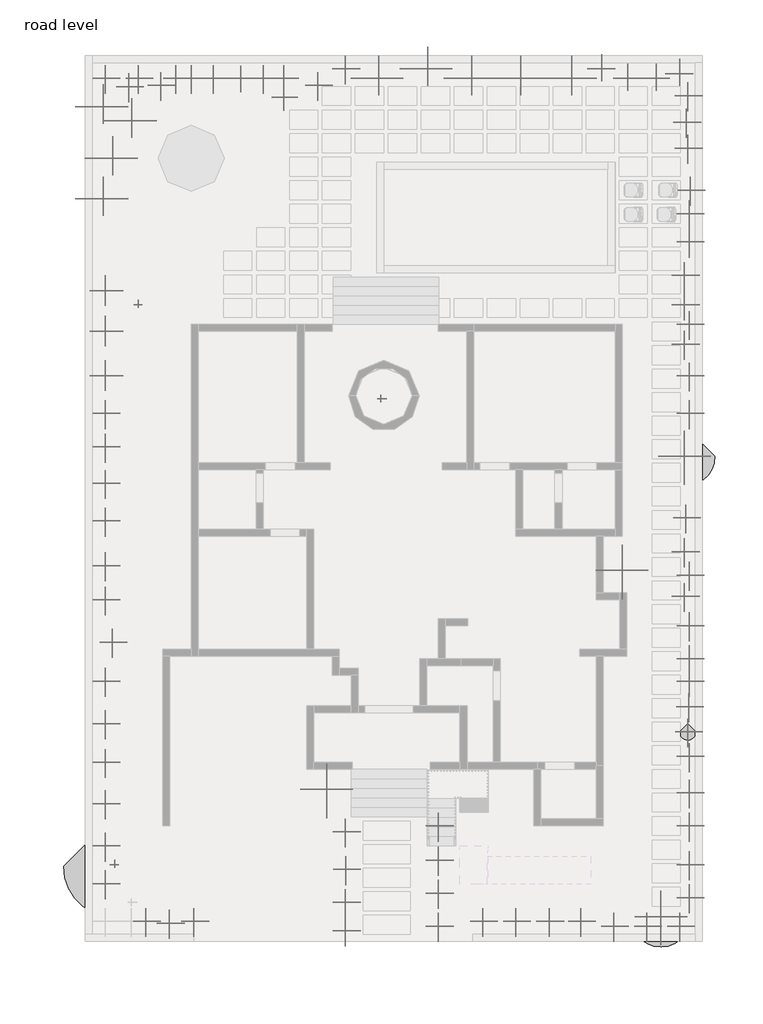
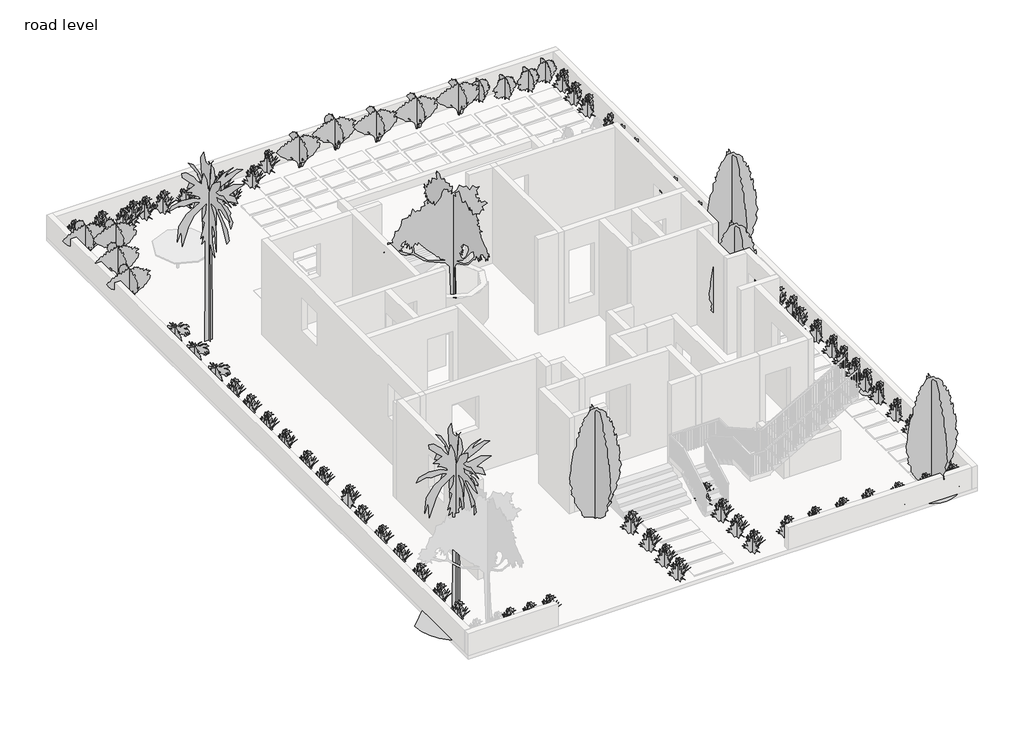
# One storey, part 5 of 5: 93 geographic elements.
"""IFC4 building model written with IfcOpenShell, lengths in millimetres."""

from ifc_helpers import new_model, si_unit, origin, place, context, project, spatial, transform, mapped, element, save
from components import rpc_plant_tropical_55f6ff97, rpc_plant_tropical_6475341c, rpc_plant_tropical_dagger_2_80c14bd7, rpc_plant_tropical_japanese_fern_2_5_30b4c15b, rpc_plant_tropical_jungle_flame_3_9c4808c2, rpc_tree_deciduous_japanese_cherry_15_bc05297b, rpc_tree_tropical_cuban_royal_palm_25_6f0ceb55, rpc_tree_tropical_grass_palm_18_ffc4a38a

model = new_model("IFC4")

# Units and contexts
model_context = context("Model", 3, world=origin())
ifc_project = project(units=[si_unit("LENGTHUNIT", "METRE", prefix="MILLI")], contexts=[model_context])

# Site, building, storey
site = spatial("IfcSite", under=ifc_project)
building = spatial("IfcBuilding", under=site)
storey = spatial("IfcBuildingStorey", under=building, Name="road level", Elevation=0.0)

# Geographic elements
placement = place(None, origin())
rpc_plant_tropical_shape = rpc_plant_tropical_55f6ff97(model_context)
element("IfcGeographicElement", 1, ObjectType="RPC Plant - Tropical", at=placement, inside=storey, context=model_context, shape_type="MappedRepresentation", body=[
    mapped(rpc_plant_tropical_shape, transform((-4250.8487175, 22497.1906886, 0.0), x_axis=(1.0, 0.0, 0.0), y_axis=(0.0, 1.0, 0.0), z_axis=(0.0, 0.0, 1.0))),
])
element("IfcGeographicElement", 2, ObjectType="RPC Plant - Tropical", at=placement, inside=storey, context=model_context, shape_type="MappedRepresentation", body=[
    mapped(rpc_plant_tropical_shape, transform((-3184.0487175, 22497.1906886, 0.0), x_axis=(1.0, 0.0, 0.0), y_axis=(0.0, 1.0, 0.0), z_axis=(0.0, 0.0, 1.0))),
])
element("IfcGeographicElement", 3, ObjectType="RPC Plant - Tropical", at=placement, inside=storey, context=model_context, shape_type="MappedRepresentation", body=[
    mapped(rpc_plant_tropical_shape, transform((-1964.8487175, 22497.1906886, 0.0), x_axis=(1.0, 0.0, 0.0), y_axis=(0.0, 1.0, 0.0), z_axis=(0.0, 0.0, 1.0))),
])
element("IfcGeographicElement", 4, ObjectType="RPC Plant - Tropical", at=placement, inside=storey, context=model_context, shape_type="MappedRepresentation", body=[
    mapped(rpc_plant_tropical_shape, transform((1530.4394971, 22497.1906886, 0.0), x_axis=(1.0, 0.0, 0.0), y_axis=(0.0, 1.0, 0.0), z_axis=(0.0, 0.0, 1.0))),
])
element("IfcGeographicElement", 5, ObjectType="RPC Plant - Tropical", at=placement, inside=storey, context=model_context, shape_type="MappedRepresentation", body=[
    mapped(rpc_plant_tropical_shape, transform((3511.6394971, 22801.9906886, 0.0), x_axis=(1.0, 0.0, 0.0), y_axis=(0.0, 1.0, 0.0), z_axis=(0.0, 0.0, 1.0))),
])
element("IfcGeographicElement", 6, ObjectType="RPC Plant - Tropical", at=placement, inside=storey, context=model_context, shape_type="MappedRepresentation", body=[
    mapped(rpc_plant_tropical_shape, transform((2630.2047352, 22268.5906886, 0.0), x_axis=(1.0, 0.0, 0.0), y_axis=(0.0, 1.0, 0.0), z_axis=(0.0, 0.0, 1.0))),
])
element("IfcGeographicElement", 7, ObjectType="RPC Plant - Tropical", at=placement, inside=storey, context=model_context, shape_type="MappedRepresentation", body=[
    mapped(rpc_plant_tropical_shape, transform((867.2512825, 22497.1906886, 0.0), x_axis=(1.0, 0.0, 0.0), y_axis=(0.0, 1.0, 0.0), z_axis=(0.0, 0.0, 1.0))),
])
element("IfcGeographicElement", 8, ObjectType="RPC Plant - Tropical", at=placement, inside=storey, context=model_context, shape_type="MappedRepresentation", body=[
    mapped(rpc_plant_tropical_shape, transform((-755.5605029, 22497.1906886, 0.0), x_axis=(1.0, 0.0, 0.0), y_axis=(0.0, 1.0, 0.0), z_axis=(0.0, 0.0, 1.0))),
])
element("IfcGeographicElement", 9, ObjectType="RPC Plant - Tropical", at=placement, inside=storey, context=model_context, shape_type="MappedRepresentation", body=[
    mapped(rpc_plant_tropical_shape, transform((-1469.5487175, 22497.1906886, 0.0), x_axis=(1.0, 0.0, 0.0), y_axis=(0.0, 1.0, 0.0), z_axis=(0.0, 0.0, 1.0))),
])
element("IfcGeographicElement", 10, ObjectType="RPC Plant - Tropical", at=placement, inside=storey, context=model_context, shape_type="MappedRepresentation", body=[
    mapped(rpc_plant_tropical_shape, transform((-2459.5797144, 22268.5906886, 0.0), x_axis=(1.0, 0.0, 0.0), y_axis=(0.0, 1.0, 0.0), z_axis=(0.0, 0.0, 1.0))),
])
element("IfcGeographicElement", 11, ObjectType="RPC Plant - Tropical", at=placement, inside=storey, context=model_context, shape_type="MappedRepresentation", body=[
    mapped(rpc_plant_tropical_shape, transform((-3485.1574933, 22224.4169729, 0.0), x_axis=(1.0, 0.0, 0.0), y_axis=(0.0, 1.0, 0.0), z_axis=(0.0, 0.0, 1.0))),
])
element("IfcGeographicElement", 12, ObjectType="RPC Plant - Tropical", at=placement, inside=storey, context=model_context, shape_type="MappedRepresentation", body=[
    mapped(rpc_plant_tropical_shape, transform((14595.9512825, 21938.3906886, 0.0), x_axis=(1.0, 0.0, 0.0), y_axis=(0.0, 1.0, 0.0), z_axis=(0.0, 0.0, 1.0))),
])
element("IfcGeographicElement", 13, ObjectType="RPC Plant - Tropical", at=placement, inside=storey, context=model_context, shape_type="MappedRepresentation", body=[
    mapped(rpc_plant_tropical_shape, transform((14545.1512825, 21074.7906886, 0.0), x_axis=(1.0, 0.0, 0.0), y_axis=(0.0, 1.0, 0.0), z_axis=(0.0, 0.0, 1.0))),
])
element("IfcGeographicElement", 14, ObjectType="RPC Plant - Tropical", at=placement, inside=storey, context=model_context, shape_type="MappedRepresentation", body=[
    mapped(rpc_plant_tropical_shape, transform((14684.8512825, 18877.6906886, 0.0), x_axis=(1.0, 0.0, 0.0), y_axis=(0.0, 1.0, 0.0), z_axis=(0.0, 0.0, 1.0))),
])
element("IfcGeographicElement", 15, ObjectType="RPC Plant - Tropical", at=placement, inside=storey, context=model_context, shape_type="MappedRepresentation", body=[
    mapped(rpc_plant_tropical_shape, transform((14646.7512825, 17201.2906886, 0.0), x_axis=(1.0, 0.0, 0.0), y_axis=(0.0, 1.0, 0.0), z_axis=(0.0, 0.0, 1.0))),
])
element("IfcGeographicElement", 16, ObjectType="RPC Plant - Tropical", at=placement, inside=storey, context=model_context, shape_type="MappedRepresentation", body=[
    mapped(rpc_plant_tropical_shape, transform((14646.7512825, 18115.6906886, 0.0), x_axis=(1.0, 0.0, 0.0), y_axis=(0.0, 1.0, 0.0), z_axis=(0.0, 0.0, 1.0))),
])
element("IfcGeographicElement", 17, ObjectType="RPC Plant - Tropical", at=placement, inside=storey, context=model_context, shape_type="MappedRepresentation", body=[
    mapped(rpc_plant_tropical_shape, transform((14595.9512825, 20236.5906886, 0.0), x_axis=(1.0, 0.0, 0.0), y_axis=(0.0, 1.0, 0.0), z_axis=(0.0, 0.0, 1.0))),
])
element("IfcGeographicElement", 18, ObjectType="RPC Plant - Tropical", at=placement, inside=storey, context=model_context, shape_type="MappedRepresentation", body=[
    mapped(rpc_plant_tropical_shape, transform((14494.3512825, 16121.7906886, 0.0), x_axis=(1.0, 0.0, 0.0), y_axis=(0.0, 1.0, 0.0), z_axis=(0.0, 0.0, 1.0))),
])
element("IfcGeographicElement", 19, ObjectType="RPC Plant - Tropical", at=placement, inside=storey, context=model_context, shape_type="MappedRepresentation", body=[
    mapped(rpc_plant_tropical_shape, transform((14494.3512825, 15169.2906886, 0.0), x_axis=(1.0, 0.0, 0.0), y_axis=(0.0, 1.0, 0.0), z_axis=(0.0, 0.0, 1.0))),
])
element("IfcGeographicElement", 20, ObjectType="RPC Plant - Tropical", at=placement, inside=storey, context=model_context, shape_type="MappedRepresentation", body=[
    mapped(rpc_plant_tropical_shape, transform((14494.3512825, 13898.7232877, 0.0), x_axis=(1.0, 0.0, 0.0), y_axis=(0.0, 1.0, 0.0), z_axis=(0.0, 0.0, 1.0))),
])
element("IfcGeographicElement", 21, ObjectType="RPC Plant - Tropical", at=placement, inside=storey, context=model_context, shape_type="MappedRepresentation", body=[
    mapped(rpc_plant_tropical_shape, transform((14646.7512825, 12870.0232877, 0.0), x_axis=(1.0, 0.0, 0.0), y_axis=(0.0, 1.0, 0.0), z_axis=(0.0, 0.0, 1.0))),
])
element("IfcGeographicElement", 22, ObjectType="RPC Plant - Tropical", at=placement, inside=storey, context=model_context, shape_type="MappedRepresentation", body=[
    mapped(rpc_plant_tropical_shape, transform((14646.7512825, 11650.8232877, 0.0), x_axis=(1.0, 0.0, 0.0), y_axis=(0.0, 1.0, 0.0), z_axis=(0.0, 0.0, 1.0))),
])
element("IfcGeographicElement", 23, ObjectType="RPC Plant - Tropical", at=placement, inside=storey, context=model_context, shape_type="MappedRepresentation", body=[
    mapped(rpc_plant_tropical_shape, transform((-4250.8487175, 11650.8232877, 0.0), x_axis=(1.0, 0.0, 0.0), y_axis=(0.0, 1.0, 0.0), z_axis=(0.0, 0.0, 1.0))),
])
element("IfcGeographicElement", 24, ObjectType="RPC Plant - Tropical", at=placement, inside=storey, context=model_context, shape_type="MappedRepresentation", body=[
    mapped(rpc_plant_tropical_shape, transform((-4250.8487175, 10567.4181776, 0.0), x_axis=(1.0, 0.0, 0.0), y_axis=(0.0, 1.0, 0.0), z_axis=(0.0, 0.0, 1.0))),
])
element("IfcGeographicElement", 25, ObjectType="RPC Plant - Tropical", at=placement, inside=storey, context=model_context, shape_type="MappedRepresentation", body=[
    mapped(rpc_plant_tropical_shape, transform((-4250.8487175, 9390.7906886, 0.0), x_axis=(1.0, 0.0, 0.0), y_axis=(0.0, 1.0, 0.0), z_axis=(0.0, 0.0, 1.0))),
])
element("IfcGeographicElement", 26, ObjectType="RPC Plant - Tropical", at=placement, inside=storey, context=model_context, shape_type="MappedRepresentation", body=[
    mapped(rpc_plant_tropical_shape, transform((-4250.8487175, 8171.5906886, 0.0), x_axis=(1.0, 0.0, 0.0), y_axis=(0.0, 1.0, 0.0), z_axis=(0.0, 0.0, 1.0))),
])
element("IfcGeographicElement", 27, ObjectType="RPC Plant - Tropical", at=placement, inside=storey, context=model_context, shape_type="MappedRepresentation", body=[
    mapped(rpc_plant_tropical_shape, transform((-4250.8487175, 6723.7906886, 0.0), x_axis=(1.0, 0.0, 0.0), y_axis=(0.0, 1.0, 0.0), z_axis=(0.0, 0.0, 1.0))),
])
element("IfcGeographicElement", 28, ObjectType="RPC Plant - Tropical", at=placement, inside=storey, context=model_context, shape_type="MappedRepresentation", body=[
    mapped(rpc_plant_tropical_shape, transform((-4250.8487175, 5618.8906886, 0.0), x_axis=(1.0, 0.0, 0.0), y_axis=(0.0, 1.0, 0.0), z_axis=(0.0, 0.0, 1.0))),
])
element("IfcGeographicElement", 29, ObjectType="RPC Plant - Tropical", at=placement, inside=storey, context=model_context, shape_type="MappedRepresentation", body=[
    mapped(rpc_plant_tropical_shape, transform((-4022.2487175, 4247.2906886, 0.0), x_axis=(1.0, 0.0, 0.0), y_axis=(0.0, 1.0, 0.0), z_axis=(0.0, 0.0, 1.0))),
])
element("IfcGeographicElement", 30, ObjectType="RPC Plant - Tropical", at=placement, inside=storey, context=model_context, shape_type="MappedRepresentation", body=[
    mapped(rpc_plant_tropical_shape, transform((-4250.8487175, 2989.9906886, 0.0), x_axis=(1.0, 0.0, 0.0), y_axis=(0.0, 1.0, 0.0), z_axis=(0.0, 0.0, 1.0))),
])
element("IfcGeographicElement", 31, ObjectType="RPC Plant - Tropical", at=placement, inside=storey, context=model_context, shape_type="MappedRepresentation", body=[
    mapped(rpc_plant_tropical_shape, transform((-4250.8487175, 1618.3906886, 0.0), x_axis=(1.0, 0.0, 0.0), y_axis=(0.0, 1.0, 0.0), z_axis=(0.0, 0.0, 1.0))),
])
element("IfcGeographicElement", 32, ObjectType="RPC Plant - Tropical", at=placement, inside=storey, context=model_context, shape_type="MappedRepresentation", body=[
    mapped(rpc_plant_tropical_shape, transform((-4250.8487175, 361.0906886, 0.0), x_axis=(1.0, 0.0, 0.0), y_axis=(0.0, 1.0, 0.0), z_axis=(0.0, 0.0, 1.0))),
])
element("IfcGeographicElement", 33, ObjectType="RPC Plant - Tropical", at=placement, inside=storey, context=model_context, shape_type="MappedRepresentation", body=[
    mapped(rpc_plant_tropical_shape, transform((-4250.8487175, -972.4093114, 0.0), x_axis=(1.0, 0.0, 0.0), y_axis=(0.0, 1.0, 0.0), z_axis=(0.0, 0.0, 1.0))),
])
element("IfcGeographicElement", 34, ObjectType="RPC Plant - Tropical", at=placement, inside=storey, context=model_context, shape_type="MappedRepresentation", body=[
    mapped(rpc_plant_tropical_shape, transform((-4250.8487175, -2344.0093114, 0.0), x_axis=(1.0, 0.0, 0.0), y_axis=(0.0, 1.0, 0.0), z_axis=(0.0, 0.0, 1.0))),
])
element("IfcGeographicElement", 35, ObjectType="RPC Plant - Tropical", at=placement, inside=storey, context=model_context, shape_type="MappedRepresentation", body=[
    mapped(rpc_plant_tropical_shape, transform((-4250.8487175, -3563.2093114, 0.0), x_axis=(1.0, 0.0, 0.0), y_axis=(0.0, 1.0, 0.0), z_axis=(0.0, 0.0, 1.0))),
])
element("IfcGeographicElement", 36, ObjectType="RPC Plant - Tropical", at=placement, inside=storey, context=model_context, shape_type="MappedRepresentation", body=[
    mapped(rpc_plant_tropical_shape, transform((11141.5512825, -4782.4093114, 0.0), x_axis=(1.0, 0.0, 0.0), y_axis=(0.0, 1.0, 0.0), z_axis=(0.0, 0.0, 1.0))),
])
element("IfcGeographicElement", 37, ObjectType="RPC Plant - Tropical", at=placement, inside=storey, context=model_context, shape_type="MappedRepresentation", body=[
    mapped(rpc_plant_tropical_shape, transform((12208.3512825, -4934.8093114, 0.0), x_axis=(1.0, 0.0, 0.0), y_axis=(0.0, 1.0, 0.0), z_axis=(0.0, 0.0, 1.0))),
])
element("IfcGeographicElement", 38, ObjectType="RPC Plant - Tropical", at=placement, inside=storey, context=model_context, shape_type="MappedRepresentation", body=[
    mapped(rpc_plant_tropical_shape, transform((13275.1512825, -4934.8093114, 0.0), x_axis=(1.0, 0.0, 0.0), y_axis=(0.0, 1.0, 0.0), z_axis=(0.0, 0.0, 1.0))),
])
element("IfcGeographicElement", 39, ObjectType="RPC Plant - Tropical", at=placement, inside=storey, context=model_context, shape_type="MappedRepresentation", body=[
    mapped(rpc_plant_tropical_shape, transform((14341.9512825, -4934.8093114, 0.0), x_axis=(1.0, 0.0, 0.0), y_axis=(0.0, 1.0, 0.0), z_axis=(0.0, 0.0, 1.0))),
])
element("IfcGeographicElement", 40, ObjectType="RPC Plant - Tropical", at=placement, inside=storey, context=model_context, shape_type="MappedRepresentation", body=[
    mapped(rpc_plant_tropical_shape, transform((14646.7512825, -2953.6093114, 0.0), x_axis=(1.0, 0.0, 0.0), y_axis=(0.0, 1.0, 0.0), z_axis=(0.0, 0.0, 1.0))),
])
element("IfcGeographicElement", 41, ObjectType="RPC Plant - Tropical", at=placement, inside=storey, context=model_context, shape_type="MappedRepresentation", body=[
    mapped(rpc_plant_tropical_shape, transform((14646.7512825, -4020.4093114, 0.0), x_axis=(1.0, 0.0, 0.0), y_axis=(0.0, 1.0, 0.0), z_axis=(0.0, 0.0, 1.0))),
])
element("IfcGeographicElement", 42, ObjectType="RPC Plant - Tropical", at=placement, inside=storey, context=model_context, shape_type="MappedRepresentation", body=[
    mapped(rpc_plant_tropical_shape, transform((14646.7512825, -1696.3093114, 0.0), x_axis=(1.0, 0.0, 0.0), y_axis=(0.0, 1.0, 0.0), z_axis=(0.0, 0.0, 1.0))),
])
element("IfcGeographicElement", 43, ObjectType="RPC Plant - Tropical", at=placement, inside=storey, context=model_context, shape_type="MappedRepresentation", body=[
    mapped(rpc_plant_tropical_shape, transform((14646.7512825, 551.5906886, 0.0), x_axis=(1.0, 0.0, 0.0), y_axis=(0.0, 1.0, 0.0), z_axis=(0.0, 0.0, 1.0))),
])
element("IfcGeographicElement", 44, ObjectType="RPC Plant - Tropical", at=placement, inside=storey, context=model_context, shape_type="MappedRepresentation", body=[
    mapped(rpc_plant_tropical_shape, transform((14598.0223193, 1348.3086582, 50.8), x_axis=(1.0, 0.0, 0.0), y_axis=(0.0, 1.0, 0.0), z_axis=(0.0, 0.0, 1.0))),
])
element("IfcGeographicElement", 45, ObjectType="RPC Plant - Tropical", at=placement, inside=storey, context=model_context, shape_type="MappedRepresentation", body=[
    mapped(rpc_plant_tropical_shape, transform((14646.7512825, 2989.9906886, 0.0), x_axis=(1.0, 0.0, 0.0), y_axis=(0.0, 1.0, 0.0), z_axis=(0.0, 0.0, 1.0))),
])
element("IfcGeographicElement", 46, ObjectType="RPC Plant - Tropical", at=placement, inside=storey, context=model_context, shape_type="MappedRepresentation", body=[
    mapped(rpc_plant_tropical_shape, transform((14634.0512825, 2164.4906886, 0.0), x_axis=(1.0, 0.0, 0.0), y_axis=(0.0, 1.0, 0.0), z_axis=(0.0, 0.0, 1.0))),
])
element("IfcGeographicElement", 47, ObjectType="RPC Plant - Tropical", at=placement, inside=storey, context=model_context, shape_type="MappedRepresentation", body=[
    mapped(rpc_plant_tropical_shape, transform((14646.7512825, 3713.8906886, 0.0), x_axis=(1.0, 0.0, 0.0), y_axis=(0.0, 1.0, 0.0), z_axis=(0.0, 0.0, 1.0))),
])
element("IfcGeographicElement", 48, ObjectType="RPC Plant - Tropical", at=placement, inside=storey, context=model_context, shape_type="MappedRepresentation", body=[
    mapped(rpc_plant_tropical_shape, transform((14494.3512825, 5733.1906886, 0.0), x_axis=(1.0, 0.0, 0.0), y_axis=(0.0, 1.0, 0.0), z_axis=(0.0, 0.0, 1.0))),
])
element("IfcGeographicElement", 49, ObjectType="RPC Plant - Tropical", at=placement, inside=storey, context=model_context, shape_type="MappedRepresentation", body=[
    mapped(rpc_plant_tropical_shape, transform((14494.3512825, 7180.9906886, 0.0), x_axis=(1.0, 0.0, 0.0), y_axis=(0.0, 1.0, 0.0), z_axis=(0.0, 0.0, 1.0))),
])
element("IfcGeographicElement", 50, ObjectType="RPC Plant - Tropical", at=placement, inside=storey, context=model_context, shape_type="MappedRepresentation", body=[
    mapped(rpc_plant_tropical_shape, transform((14532.4512825, 8273.1906886, 0.0), x_axis=(1.0, 0.0, 0.0), y_axis=(0.0, 1.0, 0.0), z_axis=(0.0, 0.0, 1.0))),
])
element("IfcGeographicElement", 51, ObjectType="RPC Plant - Tropical", at=placement, inside=storey, context=model_context, shape_type="MappedRepresentation", body=[
    mapped(rpc_plant_tropical_shape, transform((14646.7512825, -625.9346387, 0.0), x_axis=(1.0, 0.0, 0.0), y_axis=(0.0, 1.0, 0.0), z_axis=(0.0, 0.0, 1.0))),
])
element("IfcGeographicElement", 52, ObjectType="RPC Plant - Tropical", at=placement, inside=storey, context=model_context, shape_type="MappedRepresentation", body=[
    mapped(rpc_plant_tropical_shape, transform((14646.7512825, 4780.6906886, 0.0), x_axis=(1.0, 0.0, 0.0), y_axis=(0.0, 1.0, 0.0), z_axis=(0.0, 0.0, 1.0))),
])
element("IfcGeographicElement", 53, ObjectType="RPC Plant - Tropical", at=placement, inside=storey, context=model_context, shape_type="MappedRepresentation", body=[
    mapped(rpc_plant_tropical_shape, transform((14646.7512825, 6418.9906886, 0.0), x_axis=(1.0, 0.0, 0.0), y_axis=(0.0, 1.0, 0.0), z_axis=(0.0, 0.0, 1.0))),
])
element("IfcGeographicElement", 54, ObjectType="RPC Plant - Tropical", at=placement, inside=storey, context=model_context, shape_type="MappedRepresentation", body=[
    mapped(rpc_plant_tropical_shape, transform((14646.7512825, 14534.2906886, 0.0), x_axis=(1.0, 0.0, 0.0), y_axis=(0.0, 1.0, 0.0), z_axis=(0.0, 0.0, 1.0))),
])
element("IfcGeographicElement", 55, ObjectType="RPC Plant - Tropical", at=placement, inside=storey, context=model_context, shape_type="MappedRepresentation", body=[
    mapped(rpc_plant_tropical_shape, transform((3521.5512825, -1886.8093114, 0.0), x_axis=(1.0, 0.0, 0.0), y_axis=(0.0, 1.0, 0.0), z_axis=(0.0, 0.0, 1.0))),
])
element("IfcGeographicElement", 56, ObjectType="RPC Plant - Tropical", at=placement, inside=storey, context=model_context, shape_type="MappedRepresentation", body=[
    mapped(rpc_plant_tropical_shape, transform((3534.2512825, -3106.0093114, 0.0), x_axis=(1.0, 0.0, 0.0), y_axis=(0.0, 1.0, 0.0), z_axis=(0.0, 0.0, 1.0))),
])
element("IfcGeographicElement", 57, ObjectType="RPC Plant - Tropical", at=placement, inside=storey, context=model_context, shape_type="MappedRepresentation", body=[
    mapped(rpc_plant_tropical_shape, transform((3521.5512825, -4172.8093114, 0.0), x_axis=(1.0, 0.0, 0.0), y_axis=(0.0, 1.0, 0.0), z_axis=(0.0, 0.0, 1.0))),
])
element("IfcGeographicElement", 58, ObjectType="RPC Plant - Tropical", at=placement, inside=storey, context=model_context, shape_type="MappedRepresentation", body=[
    mapped(rpc_plant_tropical_shape, transform((3521.5512825, -5087.2093114, 0.0), x_axis=(1.0, 0.0, 0.0), y_axis=(0.0, 1.0, 0.0), z_axis=(0.0, 0.0, 1.0))),
])
element("IfcGeographicElement", 59, ObjectType="RPC Plant - Tropical", at=placement, inside=storey, context=model_context, shape_type="MappedRepresentation", body=[
    mapped(rpc_plant_tropical_shape, transform((6531.4512825, -1696.3093114, 0.0), x_axis=(1.0, 0.0, 0.0), y_axis=(0.0, 1.0, 0.0), z_axis=(0.0, 0.0, 1.0))),
])
element("IfcGeographicElement", 60, ObjectType="RPC Plant - Tropical", at=placement, inside=storey, context=model_context, shape_type="MappedRepresentation", body=[
    mapped(rpc_plant_tropical_shape, transform((6531.4512825, -2801.2093114, 0.0), x_axis=(1.0, 0.0, 0.0), y_axis=(0.0, 1.0, 0.0), z_axis=(0.0, 0.0, 1.0))),
])
element("IfcGeographicElement", 61, ObjectType="RPC Plant - Tropical", at=placement, inside=storey, context=model_context, shape_type="MappedRepresentation", body=[
    mapped(rpc_plant_tropical_shape, transform((6531.4512825, -3868.0093114, 0.0), x_axis=(1.0, 0.0, 0.0), y_axis=(0.0, 1.0, 0.0), z_axis=(0.0, 0.0, 1.0))),
])
element("IfcGeographicElement", 62, ObjectType="RPC Plant - Tropical", at=placement, inside=storey, context=model_context, shape_type="MappedRepresentation", body=[
    mapped(rpc_plant_tropical_shape, transform((6531.4512825, -4934.8093114, 0.0), x_axis=(1.0, 0.0, 0.0), y_axis=(0.0, 1.0, 0.0), z_axis=(0.0, 0.0, 1.0))),
])
element("IfcGeographicElement", 63, ObjectType="RPC Plant - Tropical", at=placement, inside=storey, context=model_context, shape_type="MappedRepresentation", body=[
    mapped(rpc_plant_tropical_shape, transform((10112.8512825, -4782.4093114, 0.0), x_axis=(1.0, 0.0, 0.0), y_axis=(0.0, 1.0, 0.0), z_axis=(0.0, 0.0, 1.0))),
])
element("IfcGeographicElement", 64, ObjectType="RPC Plant - Tropical", at=placement, inside=storey, context=model_context, shape_type="MappedRepresentation", body=[
    mapped(rpc_plant_tropical_shape, transform((9033.3512825, -4782.4093114, 0.0), x_axis=(1.0, 0.0, 0.0), y_axis=(0.0, 1.0, 0.0), z_axis=(0.0, 0.0, 1.0))),
])
element("IfcGeographicElement", 65, ObjectType="RPC Plant - Tropical", at=placement, inside=storey, context=model_context, shape_type="MappedRepresentation", body=[
    mapped(rpc_plant_tropical_shape, transform((7966.5512825, -4782.4093114, 0.0), x_axis=(1.0, 0.0, 0.0), y_axis=(0.0, 1.0, 0.0), z_axis=(0.0, 0.0, 1.0))),
])
element("IfcGeographicElement", 66, ObjectType="RPC Plant - Tropical", at=placement, inside=storey, context=model_context, shape_type="MappedRepresentation", body=[
    mapped(rpc_plant_tropical_shape, transform((-2171.3661488, -4843.5212079, 0.0), x_axis=(1.0, 0.0, 0.0), y_axis=(0.0, 1.0, 0.0), z_axis=(0.0, 0.0, 1.0))),
])
element("IfcGeographicElement", 67, ObjectType="RPC Plant - Tropical", at=placement, inside=storey, context=model_context, shape_type="MappedRepresentation", body=[
    mapped(rpc_plant_tropical_shape, transform((-2939.5165353, -4783.8107175, 0.0), x_axis=(1.0, 0.0, 0.0), y_axis=(0.0, 1.0, 0.0), z_axis=(0.0, 0.0, 1.0))),
])
element("IfcGeographicElement", 68, ObjectType="RPC Plant - Tropical", at=placement, inside=storey, context=model_context, shape_type="MappedRepresentation", body=[
    mapped(rpc_plant_tropical_shape, transform((-1380.6487175, -4782.4093114, 0.0), x_axis=(1.0, 0.0, 0.0), y_axis=(0.0, 1.0, 0.0), z_axis=(0.0, 0.0, 1.0))),
])
rpc_plant_tropical_2_shape = rpc_plant_tropical_6475341c(model_context)
element("IfcGeographicElement", 69, ObjectType="RPC Plant - Tropical", at=placement, inside=storey, context=model_context, shape_type="MappedRepresentation", body=[
    mapped(rpc_plant_tropical_2_shape, transform((4654.6394971, 22497.1906886, 0.0), x_axis=(1.0, 0.0, 0.0), y_axis=(0.0, 1.0, 0.0), z_axis=(0.0, 0.0, 1.0))),
])
element("IfcGeographicElement", 70, ObjectType="RPC Plant - Tropical", at=placement, inside=storey, context=model_context, shape_type="MappedRepresentation", body=[
    mapped(rpc_plant_tropical_2_shape, transform((7674.4512825, 22497.1906886, 0.0), x_axis=(1.0, 0.0, 0.0), y_axis=(0.0, 1.0, 0.0), z_axis=(0.0, 0.0, 1.0))),
])
element("IfcGeographicElement", 71, ObjectType="RPC Plant - Tropical", at=placement, inside=storey, context=model_context, shape_type="MappedRepresentation", body=[
    mapped(rpc_plant_tropical_2_shape, transform((6239.3512825, 22801.9906886, 0.0), x_axis=(1.0, 0.0, 0.0), y_axis=(0.0, 1.0, 0.0), z_axis=(0.0, 0.0, 1.0))),
])
element("IfcGeographicElement", 72, ObjectType="RPC Plant - Tropical", at=placement, inside=storey, context=model_context, shape_type="MappedRepresentation", body=[
    mapped(rpc_plant_tropical_2_shape, transform((9261.9512825, 22497.1906886, 0.0), x_axis=(1.0, 0.0, 0.0), y_axis=(0.0, 1.0, 0.0), z_axis=(0.0, 0.0, 1.0))),
])
element("IfcGeographicElement", 73, ObjectType="RPC Plant - Tropical", at=placement, inside=storey, context=model_context, shape_type="MappedRepresentation", body=[
    mapped(rpc_plant_tropical_2_shape, transform((10903.0394971, 22497.1906886, 0.0), x_axis=(1.0, 0.0, 0.0), y_axis=(0.0, 1.0, 0.0), z_axis=(0.0, 0.0, 1.0))),
])
element("IfcGeographicElement", 74, ObjectType="RPC Plant - Tropical", at=placement, inside=storey, context=model_context, shape_type="MappedRepresentation", body=[
    mapped(rpc_plant_tropical_2_shape, transform((-4250.8487175, 21582.7906886, 0.0), x_axis=(1.0, 0.0, 0.0), y_axis=(0.0, 1.0, 0.0), z_axis=(0.0, 0.0, 1.0))),
])
element("IfcGeographicElement", 75, ObjectType="RPC Plant - Tropical", at=placement, inside=storey, context=model_context, shape_type="MappedRepresentation", body=[
    mapped(rpc_plant_tropical_2_shape, transform((-3946.0487175, 19906.3906886, 0.0), x_axis=(1.0, 0.0, 0.0), y_axis=(0.0, 1.0, 0.0), z_axis=(0.0, 0.0, 1.0))),
])
element("IfcGeographicElement", 76, ObjectType="RPC Plant - Tropical", at=placement, inside=storey, context=model_context, shape_type="MappedRepresentation", body=[
    mapped(rpc_plant_tropical_2_shape, transform((-4250.8487175, 18594.9545816, 0.0), x_axis=(1.0, 0.0, 0.0), y_axis=(0.0, 1.0, 0.0), z_axis=(0.0, 0.0, 1.0))),
])
element("IfcGeographicElement", 77, ObjectType="RPC Plant - Tropical", at=placement, inside=storey, context=model_context, shape_type="MappedRepresentation", body=[
    mapped(rpc_plant_tropical_2_shape, transform((-3332.7574933, 21125.5906886, 0.0), x_axis=(1.0, 0.0, 0.0), y_axis=(0.0, 1.0, 0.0), z_axis=(0.0, 0.0, 1.0))),
])
rpc_plant_tropical_dagger_2_shape = rpc_plant_tropical_dagger_2_80c14bd7(model_context)
element("IfcGeographicElement", 78, ObjectType="RPC Plant - Tropical : Dagger - 2'", at=placement, inside=storey, context=model_context, shape_type="MappedRepresentation", body=[
    mapped(rpc_plant_tropical_dagger_2_shape, transform((143.3512825, 22497.1906886, 0.0), x_axis=(1.0, 0.0, 0.0), y_axis=(0.0, 1.0, 0.0), z_axis=(0.0, 0.0, 1.0))),
])
element("IfcGeographicElement", 79, ObjectType="RPC Plant - Tropical : Dagger - 2'", at=placement, inside=storey, context=model_context, shape_type="MappedRepresentation", body=[
    mapped(rpc_plant_tropical_dagger_2_shape, transform((1530.4394971, 21887.5906886, 0.0), x_axis=(1.0, 0.0, 0.0), y_axis=(0.0, 1.0, 0.0), z_axis=(0.0, 0.0, 1.0))),
])
rpc_plant_tropical_japanese_fern_2_5_shape = rpc_plant_tropical_japanese_fern_2_5_30b4c15b(model_context)
element("IfcGeographicElement", 80, ObjectType="RPC Plant - Tropical : Japanese Fern - 2.5'", at=placement, inside=storey, context=model_context, shape_type="MappedRepresentation", body=[
    mapped(rpc_plant_tropical_japanese_fern_2_5_shape, transform((-4250.8487175, 15626.4906886, 0.0), x_axis=(1.0, 0.0, 0.0), y_axis=(0.0, 1.0, 0.0), z_axis=(0.0, 0.0, 1.0))),
])
element("IfcGeographicElement", 81, ObjectType="RPC Plant - Tropical : Japanese Fern - 2.5'", at=placement, inside=storey, context=model_context, shape_type="MappedRepresentation", body=[
    mapped(rpc_plant_tropical_japanese_fern_2_5_shape, transform((-4250.8487175, 14305.6906886, 0.0), x_axis=(1.0, 0.0, 0.0), y_axis=(0.0, 1.0, 0.0), z_axis=(0.0, 0.0, 1.0))),
])
element("IfcGeographicElement", 82, ObjectType="RPC Plant - Tropical : Japanese Fern - 2.5'", at=placement, inside=storey, context=model_context, shape_type="MappedRepresentation", body=[
    mapped(rpc_plant_tropical_japanese_fern_2_5_shape, transform((-4250.8487175, 12870.0232877, 0.0), x_axis=(1.0, 0.0, 0.0), y_axis=(0.0, 1.0, 0.0), z_axis=(0.0, 0.0, 1.0))),
])
rpc_plant_tropical_jungle_flame_3_shape = rpc_plant_tropical_jungle_flame_3_9c4808c2(model_context)
element("IfcGeographicElement", 83, ObjectType="RPC Plant - Tropical : Jungle Flame - 3'", at=placement, inside=storey, context=model_context, shape_type="MappedRepresentation", body=[
    mapped(rpc_plant_tropical_jungle_flame_3_shape, transform((11817.4394971, 22801.9906886, 0.0), x_axis=(1.0, 0.0, 0.0), y_axis=(0.0, 1.0, 0.0), z_axis=(0.0, 0.0, 1.0))),
])
element("IfcGeographicElement", 84, ObjectType="RPC Plant - Tropical : Jungle Flame - 3'", at=placement, inside=storey, context=model_context, shape_type="MappedRepresentation", body=[
    mapped(rpc_plant_tropical_jungle_flame_3_shape, transform((12665.5512825, 22497.1906886, 0.0), x_axis=(1.0, 0.0, 0.0), y_axis=(0.0, 1.0, 0.0), z_axis=(0.0, 0.0, 1.0))),
])
element("IfcGeographicElement", 85, ObjectType="RPC Plant - Tropical : Jungle Flame - 3'", at=placement, inside=storey, context=model_context, shape_type="MappedRepresentation", body=[
    mapped(rpc_plant_tropical_jungle_flame_3_shape, transform((14341.9512825, 22649.5906886, 0.0), x_axis=(1.0, 0.0, 0.0), y_axis=(0.0, 1.0, 0.0), z_axis=(0.0, 0.0, 1.0))),
])
element("IfcGeographicElement", 86, ObjectType="RPC Plant - Tropical : Jungle Flame - 3'", at=placement, inside=storey, context=model_context, shape_type="MappedRepresentation", body=[
    mapped(rpc_plant_tropical_jungle_flame_3_shape, transform((13579.9512825, 22497.1906886, 0.0), x_axis=(1.0, 0.0, 0.0), y_axis=(0.0, 1.0, 0.0), z_axis=(0.0, 0.0, 1.0))),
])
rpc_tree_deciduous_japanese_cherry_15_shape = rpc_tree_deciduous_japanese_cherry_15_bc05297b(model_context)
element("IfcGeographicElement", 87, ObjectType="RPC Tree - Deciduous : Japanese Cherry - 15'", at=placement, inside=storey, context=model_context, shape_type="MappedRepresentation", body=[
    mapped(rpc_tree_deciduous_japanese_cherry_15_shape, transform((14494.3512825, 10267.0906886, 0.0), x_axis=(1.0, 0.0, 0.0), y_axis=(0.0, 1.0, 0.0), z_axis=(0.0, 0.0, 1.0))),
])
element("IfcGeographicElement", 88, ObjectType="RPC Tree - Deciduous : Japanese Cherry - 15'", at=placement, inside=storey, context=model_context, shape_type="MappedRepresentation", body=[
    mapped(rpc_tree_deciduous_japanese_cherry_15_shape, transform((12475.0512825, 6571.3906886, 0.0), x_axis=(1.0, 0.0, 0.0), y_axis=(0.0, 1.0, 0.0), z_axis=(0.0, 0.0, 1.0))),
])
element("IfcGeographicElement", 89, ObjectType="RPC Tree - Deciduous : Japanese Cherry - 15'", at=placement, inside=storey, context=model_context, shape_type="MappedRepresentation", body=[
    mapped(rpc_tree_deciduous_japanese_cherry_15_shape, transform((2911.9512825, -515.2093114, 0.0), x_axis=(1.0, 0.0, 0.0), y_axis=(0.0, 1.0, 0.0), z_axis=(0.0, 0.0, 1.0))),
])
element("IfcGeographicElement", 90, ObjectType="RPC Tree - Deciduous : Japanese Cherry - 15'", at=placement, inside=storey, context=model_context, shape_type="MappedRepresentation", body=[
    mapped(rpc_tree_deciduous_japanese_cherry_15_shape, transform((13732.3512825, -4630.0093114, 0.0), x_axis=(1.0, 0.0, 0.0), y_axis=(0.0, 1.0, 0.0), z_axis=(0.0, 0.0, 1.0))),
])
rpc_tree_tropical_cuban_royal_palm_25_shape = rpc_tree_tropical_cuban_royal_palm_25_6f0ceb55(model_context)
element("IfcGeographicElement", 91, ObjectType="RPC Tree - Tropical : Cuban Royal Palm - 25'", at=placement, inside=storey, context=model_context, shape_type="MappedRepresentation", body=[
    mapped(rpc_tree_tropical_cuban_royal_palm_25_shape, transform((-3946.0487175, -2953.6093114, 0.0), x_axis=(1.0, 0.0, 0.0), y_axis=(0.0, 1.0, 0.0), z_axis=(0.0, 0.0, 1.0))),
])
element("IfcGeographicElement", 92, ObjectType="RPC Tree - Tropical : Cuban Royal Palm - 25'", at=placement, inside=storey, context=model_context, shape_type="MappedRepresentation", body=[
    mapped(rpc_tree_tropical_cuban_royal_palm_25_shape, transform((-3184.0487175, 15169.2906886, 0.0), x_axis=(1.0, 0.0, 0.0), y_axis=(0.0, 1.0, 0.0), z_axis=(0.0, 0.0, 1.0))),
])
rpc_tree_tropical_grass_palm_18_shape = rpc_tree_tropical_grass_palm_18_ffc4a38a(model_context)
element("IfcGeographicElement", 93, ObjectType="RPC Tree - Tropical : Grass Palm - 18'", at=placement, inside=storey, context=model_context, shape_type="MappedRepresentation", body=[
    mapped(rpc_tree_tropical_grass_palm_18_shape, transform((4664.5512825, 12133.9906886, 0.0), x_axis=(1.0, 0.0, 0.0), y_axis=(0.0, 1.0, 0.0), z_axis=(0.0, 0.0, 1.0))),
])

save(model, "model.ifc")

# Revit data of these elements
# Type "RPC Plant - Tropical"
#   built-in parameter 1005198 = "{2, 15},{39, RPC-16-FWM5-GM7X-C67P-4000-ST1L-LVER-AU},{1, 0},{1, 0},{2, 35},{1, 8},{5, Color},{1, 0},{1, 0},{3, 0.8},{3, 0.8},{3, 0.8},{1, 8},{7, BBoxMin},{1, 0},{1, 0},{1, 0},{1, 0},{1, 0},{1, 8},{7, BBoxMax},{1, 0},{1, 0},{1, 0},{1, 0},{1, 0},{2, 11},{9, RPCTypeId},{1, 0},{1, 0},{39, RPC-16-FWM5-GM7X-C67P-4000-ST1L-LVER-AU},{1, 6},{14, RPCPlantHeight},{1, 0},{1, 0},{1, 3},{2, 11},{7, keyword},{1, 0},{1, 0},{99, :Geometry:RPC:Crane Lily:strelitzia:reinae:crane lily:plants:shrub:flower:tropical:bird-of-paradise},{2, 11},{8, category},{1, 0},{1, 0},{17, :Shrubs [General]},{2, 11},{12, LocalizedUID},{1, 0},{1, 0},{10, Crane Lily},{2, 14},{6, Height},{1, 0},{1, 0},{1, 3},{1, 2},{16, Cast Reflections},{1, 0},{1, 0},{1, 0},{1, 2},{12, Cast Shadows},{1, 0},{1, 0},{1, 1},{1, 2},{9, Lock View},{1, 0},{1, 0},{1, 0},{1, 4},{5, ViewC},{1, 0},{1, 0},{1, 0},{2, 11},{20, AdvancedUIDefinition},{1, 0},{1, 0},{0, },{2, 11},{10, AssetLibID},{1, 0},{1, 0},{36, 4D3F6E72-3F99-4203-98E9-AF80B3C7A7A4},{2, 11},{10, BaseSchema},{1, 0},{1, 0},{9, RPCSchema},{2, 11},{12, ExchangeGUID},{1, 0},{1, 0},{0, },{1, 2},{6, Hidden},{1, 0},{1, 0},{1, 0},{1, 4},{11, RPCCategory},{1, 0},{1, 0},{1, 0},{2, 11},{8, RPCImage},{1, 0},{1, 0},{0, },{1, 4},{13, SchemaVersion},{1, 0},{1, 0},{1, 4},{2, 11},{12, UIDefinition},{1, 0},{1, 0},{0, },{2, 11},{6, UIName},{1, 0},{1, 0},{39, RPC-16-FWM5-GM7X-C67P-4000-ST1L-LVER-AU},{2, 11},{11, VersionGUID},{1, 0},{1, 0},{9, RPCSchema},{2, 11},{9, assettype},{1, 0},{1, 0},{11, RPCGeometry},{2, 11},{11, description},{1, 0},{1, 0},{0, },{2, 11},{9, localname},{1, 0},{1, 0},{3, RPC},{2, 11},{9, localtype},{1, 0},{1, 0},{3, RPC},{1, 4},{8, revision},{1, 0},{1, 0},{1, 1},{2, 11},{9, thumbnail},{1, 0},{1, 0},{0, },{1, 4},{7, version},{1, 0},{1, 0},{1, 1},{1, 2},{20, RPC_Cast Reflections},{1, 0},{1, 0},{1, 1},{1, 2},{16, RPC_Cast Shadows},{1, 0},{1, 0},{1, 1},{1, 2},{13, RPC_Lock View},{1, 0},{1, 0},{1, 0},{1, 4},{9, RPC_ViewC},{1, 0},{1, 0},{1, 0},{21, assetlibrary_base.fbx},{1, 5},"
#   built-in parameter 1005195 = "RPC-16-FWM5-GM7X-C67P-4000-ST1L-LVER-AU"
#   Assembly Code = "G2050500"
#   Height = 3' - 0"
#   Default Elevation = 0
# Type "RPC Plant - Tropical"
#   built-in parameter 1005198 = "{2, 15},{39, RPC-16-G3GK-N2Q0-PN0G-6000-ST1L-LVER-AU},{1, 0},{1, 0},{2, 35},{1, 8},{5, Color},{1, 0},{1, 0},{3, 0.8},{3, 0.8},{3, 0.8},{1, 8},{7, BBoxMin},{1, 0},{1, 0},{1, 0},{1, 0},{1, 0},{1, 8},{7, BBoxMax},{1, 0},{1, 0},{1, 0},{1, 0},{1, 0},{2, 11},{9, RPCTypeId},{1, 0},{1, 0},{39, RPC-16-G3GK-N2Q0-PN0G-6000-ST1L-LVER-AU},{1, 6},{14, RPCPlantHeight},{1, 0},{1, 0},{3, 4.5},{2, 11},{7, keyword},{1, 0},{1, 0},{80, :Geometry:RPC:Honey Myrtle:honey myrtle:melaleuca spathulata:tropical:austrailia},{2, 11},{8, category},{1, 0},{1, 0},{17, :Shrubs [General]},{2, 11},{12, LocalizedUID},{1, 0},{1, 0},{12, Honey Myrtle},{2, 14},{6, Height},{1, 0},{1, 0},{3, 4.5},{1, 2},{16, Cast Reflections},{1, 0},{1, 0},{1, 0},{1, 2},{12, Cast Shadows},{1, 0},{1, 0},{1, 1},{1, 2},{9, Lock View},{1, 0},{1, 0},{1, 0},{1, 4},{5, ViewC},{1, 0},{1, 0},{1, 0},{2, 11},{20, AdvancedUIDefinition},{1, 0},{1, 0},{0, },{2, 11},{10, AssetLibID},{1, 0},{1, 0},{36, 4D3F6E72-3F99-4203-98E9-AF80B3C7A7A4},{2, 11},{10, BaseSchema},{1, 0},{1, 0},{9, RPCSchema},{2, 11},{12, ExchangeGUID},{1, 0},{1, 0},{0, },{1, 2},{6, Hidden},{1, 0},{1, 0},{1, 0},{1, 4},{11, RPCCategory},{1, 0},{1, 0},{1, 0},{2, 11},{8, RPCImage},{1, 0},{1, 0},{0, },{1, 4},{13, SchemaVersion},{1, 0},{1, 0},{1, 4},{2, 11},{12, UIDefinition},{1, 0},{1, 0},{0, },{2, 11},{6, UIName},{1, 0},{1, 0},{39, RPC-16-G3GK-N2Q0-PN0G-6000-ST1L-LVER-AU},{2, 11},{11, VersionGUID},{1, 0},{1, 0},{9, RPCSchema},{2, 11},{9, assettype},{1, 0},{1, 0},{11, RPCGeometry},{2, 11},{11, description},{1, 0},{1, 0},{0, },{2, 11},{9, localname},{1, 0},{1, 0},{3, RPC},{2, 11},{9, localtype},{1, 0},{1, 0},{3, RPC},{1, 4},{8, revision},{1, 0},{1, 0},{1, 1},{2, 11},{9, thumbnail},{1, 0},{1, 0},{0, },{1, 4},{7, version},{1, 0},{1, 0},{1, 1},{1, 2},{20, RPC_Cast Reflections},{1, 0},{1, 0},{1, 1},{1, 2},{16, RPC_Cast Shadows},{1, 0},{1, 0},{1, 1},{1, 2},{13, RPC_Lock View},{1, 0},{1, 0},{1, 0},{1, 4},{9, RPC_ViewC},{1, 0},{1, 0},{1, 0},{21, assetlibrary_base.fbx},{1, 5},"
#   built-in parameter 1005195 = "RPC-16-G3GK-N2Q0-PN0G-6000-ST1L-LVER-AU"
#   Assembly Code = "G2050500"
#   Height = 4' - 6"
#   Default Elevation = 0
# Type "RPC Plant - Tropical : Dagger - 2'"
#   built-in parameter 1005198 = "{2, 15},{39, RPC-16-G3A7-NEG0-UH6H-J000-ST1L-LVER-AU},{1, 0},{1, 0},{2, 35},{1, 8},{5, Color},{1, 0},{1, 0},{3, 0.8},{3, 0.8},{3, 0.8},{1, 8},{7, BBoxMin},{1, 0},{1, 0},{1, 0},{1, 0},{1, 0},{1, 8},{7, BBoxMax},{1, 0},{1, 0},{1, 0},{1, 0},{1, 0},{2, 11},{9, RPCTypeId},{1, 0},{1, 0},{39, RPC-16-G3A7-NEG0-UH6H-J000-ST1L-LVER-AU},{1, 6},{14, RPCPlantHeight},{1, 0},{1, 0},{1, 2},{2, 11},{7, keyword},{1, 0},{1, 0},{55, :Geometry:RPC:Dagger:Yucca Recurvifolia:plant:tropical.},{2, 11},{8, category},{1, 0},{1, 0},{17, :Plants [General]},{2, 11},{12, LocalizedUID},{1, 0},{1, 0},{6, Dagger},{2, 14},{6, Height},{1, 0},{1, 0},{1, 2},{1, 2},{16, Cast Reflections},{1, 0},{1, 0},{1, 0},{1, 2},{12, Cast Shadows},{1, 0},{1, 0},{1, 1},{1, 2},{9, Lock View},{1, 0},{1, 0},{1, 0},{1, 4},{5, ViewC},{1, 0},{1, 0},{1, 0},{2, 11},{20, AdvancedUIDefinition},{1, 0},{1, 0},{0, },{2, 11},{10, AssetLibID},{1, 0},{1, 0},{36, 4D3F6E72-3F99-4203-98E9-AF80B3C7A7A4},{2, 11},{10, BaseSchema},{1, 0},{1, 0},{9, RPCSchema},{2, 11},{12, ExchangeGUID},{1, 0},{1, 0},{0, },{1, 2},{6, Hidden},{1, 0},{1, 0},{1, 0},{1, 4},{11, RPCCategory},{1, 0},{1, 0},{1, 0},{2, 11},{8, RPCImage},{1, 0},{1, 0},{0, },{1, 4},{13, SchemaVersion},{1, 0},{1, 0},{1, 4},{2, 11},{12, UIDefinition},{1, 0},{1, 0},{0, },{2, 11},{6, UIName},{1, 0},{1, 0},{39, RPC-16-G3A7-NEG0-UH6H-J000-ST1L-LVER-AU},{2, 11},{11, VersionGUID},{1, 0},{1, 0},{9, RPCSchema},{2, 11},{9, assettype},{1, 0},{1, 0},{11, RPCGeometry},{2, 11},{11, description},{1, 0},{1, 0},{0, },{2, 11},{9, localname},{1, 0},{1, 0},{3, RPC},{2, 11},{9, localtype},{1, 0},{1, 0},{3, RPC},{1, 4},{8, revision},{1, 0},{1, 0},{1, 1},{2, 11},{9, thumbnail},{1, 0},{1, 0},{0, },{1, 4},{7, version},{1, 0},{1, 0},{1, 1},{1, 2},{20, RPC_Cast Reflections},{1, 0},{1, 0},{1, 1},{1, 2},{16, RPC_Cast Shadows},{1, 0},{1, 0},{1, 1},{1, 2},{13, RPC_Lock View},{1, 0},{1, 0},{1, 0},{1, 4},{9, RPC_ViewC},{1, 0},{1, 0},{1, 0},{21, assetlibrary_base.fbx},{1, 5},"
#   built-in parameter 1005195 = "RPC-16-G3A7-NEG0-UH6H-J000-ST1L-LVER-AU"
#   Type Comments = "Dagger"
#   Assembly Code = "G2050500"
#   Height = 2' - 0"
#   Default Elevation = 0
# Type "RPC Plant - Tropical : Japanese Fern - 2.5'"
#   built-in parameter 1005198 = "{2, 15},{39, RPC-16-G1GK-JAPX-7J4P-Q000-ST1L-LVER-AU},{1, 0},{1, 0},{2, 35},{1, 8},{5, Color},{1, 0},{1, 0},{3, 0.8},{3, 0.8},{3, 0.8},{1, 8},{7, BBoxMin},{1, 0},{1, 0},{1, 0},{1, 0},{1, 0},{1, 8},{7, BBoxMax},{1, 0},{1, 0},{1, 0},{1, 0},{1, 0},{2, 11},{9, RPCTypeId},{1, 0},{1, 0},{39, RPC-16-G1GK-JAPX-7J4P-Q000-ST1L-LVER-AU},{1, 6},{14, RPCPlantHeight},{1, 0},{1, 0},{3, 2.5},{2, 11},{7, keyword},{1, 0},{1, 0},{53, :Geometry:RPC:Japanese Fern:plant:small:japanese fern},{2, 11},{8, category},{1, 0},{1, 0},{17, :Shrubs [General]},{2, 11},{12, LocalizedUID},{1, 0},{1, 0},{13, Japanese Fern},{2, 14},{6, Height},{1, 0},{1, 0},{3, 2.5},{1, 2},{16, Cast Reflections},{1, 0},{1, 0},{1, 0},{1, 2},{12, Cast Shadows},{1, 0},{1, 0},{1, 1},{1, 2},{9, Lock View},{1, 0},{1, 0},{1, 0},{1, 4},{5, ViewC},{1, 0},{1, 0},{1, 0},{2, 11},{20, AdvancedUIDefinition},{1, 0},{1, 0},{0, },{2, 11},{10, AssetLibID},{1, 0},{1, 0},{36, 4D3F6E72-3F99-4203-98E9-AF80B3C7A7A4},{2, 11},{10, BaseSchema},{1, 0},{1, 0},{9, RPCSchema},{2, 11},{12, ExchangeGUID},{1, 0},{1, 0},{0, },{1, 2},{6, Hidden},{1, 0},{1, 0},{1, 0},{1, 4},{11, RPCCategory},{1, 0},{1, 0},{1, 0},{2, 11},{8, RPCImage},{1, 0},{1, 0},{0, },{1, 4},{13, SchemaVersion},{1, 0},{1, 0},{1, 4},{2, 11},{12, UIDefinition},{1, 0},{1, 0},{0, },{2, 11},{6, UIName},{1, 0},{1, 0},{39, RPC-16-G1GK-JAPX-7J4P-Q000-ST1L-LVER-AU},{2, 11},{11, VersionGUID},{1, 0},{1, 0},{9, RPCSchema},{2, 11},{9, assettype},{1, 0},{1, 0},{11, RPCGeometry},{2, 11},{11, description},{1, 0},{1, 0},{0, },{2, 11},{9, localname},{1, 0},{1, 0},{3, RPC},{2, 11},{9, localtype},{1, 0},{1, 0},{3, RPC},{1, 4},{8, revision},{1, 0},{1, 0},{1, 1},{2, 11},{9, thumbnail},{1, 0},{1, 0},{0, },{1, 4},{7, version},{1, 0},{1, 0},{1, 1},{1, 2},{20, RPC_Cast Reflections},{1, 0},{1, 0},{1, 1},{1, 2},{16, RPC_Cast Shadows},{1, 0},{1, 0},{1, 1},{1, 2},{13, RPC_Lock View},{1, 0},{1, 0},{1, 0},{1, 4},{9, RPC_ViewC},{1, 0},{1, 0},{1, 0},{21, assetlibrary_base.fbx},{1, 5},"
#   built-in parameter 1005195 = "RPC-16-G1GK-JAPX-7J4P-Q000-ST1L-LVER-AU"
#   Type Comments = "Japanese Fern"
#   Assembly Code = "G2050500"
#   Height = 2' - 6"
#   Default Elevation = 0
# Type "RPC Plant - Tropical : Jungle Flame - 3'"
#   built-in parameter 1005198 = "{2, 15},{39, RPC-16-FUVJ-JWG0-MWGK-8000-ST1L-LVER-AU},{1, 0},{1, 0},{2, 35},{1, 8},{5, Color},{1, 0},{1, 0},{3, 0.8},{3, 0.8},{3, 0.8},{1, 8},{7, BBoxMin},{1, 0},{1, 0},{1, 0},{1, 0},{1, 0},{1, 8},{7, BBoxMax},{1, 0},{1, 0},{1, 0},{1, 0},{1, 0},{2, 11},{9, RPCTypeId},{1, 0},{1, 0},{39, RPC-16-FUVJ-JWG0-MWGK-8000-ST1L-LVER-AU},{1, 6},{14, RPCPlantHeight},{1, 0},{1, 0},{1, 3},{2, 11},{7, keyword},{1, 0},{1, 0},{90, :Geometry:RPC:Jungle Flame:ixora macrothyrsa:jungle flame:bush:shrub:plant:flower:tropical},{2, 11},{8, category},{1, 0},{1, 0},{17, :Shrubs [General]},{2, 11},{12, LocalizedUID},{1, 0},{1, 0},{12, Jungle Flame},{2, 14},{6, Height},{1, 0},{1, 0},{1, 3},{1, 2},{16, Cast Reflections},{1, 0},{1, 0},{1, 0},{1, 2},{12, Cast Shadows},{1, 0},{1, 0},{1, 1},{1, 2},{9, Lock View},{1, 0},{1, 0},{1, 0},{1, 4},{5, ViewC},{1, 0},{1, 0},{1, 0},{2, 11},{20, AdvancedUIDefinition},{1, 0},{1, 0},{0, },{2, 11},{10, AssetLibID},{1, 0},{1, 0},{36, 4D3F6E72-3F99-4203-98E9-AF80B3C7A7A4},{2, 11},{10, BaseSchema},{1, 0},{1, 0},{9, RPCSchema},{2, 11},{12, ExchangeGUID},{1, 0},{1, 0},{0, },{1, 2},{6, Hidden},{1, 0},{1, 0},{1, 0},{1, 4},{11, RPCCategory},{1, 0},{1, 0},{1, 0},{2, 11},{8, RPCImage},{1, 0},{1, 0},{0, },{1, 4},{13, SchemaVersion},{1, 0},{1, 0},{1, 4},{2, 11},{12, UIDefinition},{1, 0},{1, 0},{0, },{2, 11},{6, UIName},{1, 0},{1, 0},{39, RPC-16-FUVJ-JWG0-MWGK-8000-ST1L-LVER-AU},{2, 11},{11, VersionGUID},{1, 0},{1, 0},{9, RPCSchema},{2, 11},{9, assettype},{1, 0},{1, 0},{11, RPCGeometry},{2, 11},{11, description},{1, 0},{1, 0},{0, },{2, 11},{9, localname},{1, 0},{1, 0},{3, RPC},{2, 11},{9, localtype},{1, 0},{1, 0},{3, RPC},{1, 4},{8, revision},{1, 0},{1, 0},{1, 1},{2, 11},{9, thumbnail},{1, 0},{1, 0},{0, },{1, 4},{7, version},{1, 0},{1, 0},{1, 1},{1, 2},{20, RPC_Cast Reflections},{1, 0},{1, 0},{1, 1},{1, 2},{16, RPC_Cast Shadows},{1, 0},{1, 0},{1, 1},{1, 2},{13, RPC_Lock View},{1, 0},{1, 0},{1, 0},{1, 4},{9, RPC_ViewC},{1, 0},{1, 0},{1, 0},{21, assetlibrary_base.fbx},{1, 5},"
#   built-in parameter 1005195 = "RPC-16-FUVJ-JWG0-MWGK-8000-ST1L-LVER-AU"
#   Type Comments = "Jungle Flame"
#   Assembly Code = "G2050500"
#   Height = 3' - 0"
#   Default Elevation = 0
# Type "RPC Tree - Deciduous : Japanese Cherry - 15'"
#   built-in parameter 1005195 = "RPC-16-FUM3-UUQ0-UBF0-N000-ST1L-LVER-AU"
#   Type Comments = "Japanese Cherry"
#   Assembly Code = "G2050500"
#   Height = 15' - 0"
#   Default Elevation = 0
# Type "RPC Tree - Tropical : Cuban Royal Palm - 25'"
#   built-in parameter 1005198 = "{2, 15},{39, RPC-16-FVGV-NKG0-7NHH-C000-ST1L-LVER-AU},{1, 0},{1, 0},{2, 35},{1, 8},{5, Color},{1, 0},{1, 0},{3, 0.8},{3, 0.8},{3, 0.8},{1, 8},{7, BBoxMin},{1, 0},{1, 0},{1, 0},{1, 0},{1, 0},{1, 8},{7, BBoxMax},{1, 0},{1, 0},{1, 0},{1, 0},{1, 0},{2, 11},{9, RPCTypeId},{1, 0},{1, 0},{39, RPC-16-FVGV-NKG0-7NHH-C000-ST1L-LVER-AU},{1, 6},{14, RPCPlantHeight},{1, 0},{1, 0},{2, 25},{2, 11},{7, keyword},{1, 0},{1, 0},{72, :Geometry:RPC:Cuban Royal Palm:Roystonea regia (Oreodoxa):palm:tropical.},{2, 11},{8, category},{1, 0},{1, 0},{17, :Trees [Tropical]},{2, 11},{12, LocalizedUID},{1, 0},{1, 0},{16, Cuban Royal Palm},{2, 14},{6, Height},{1, 0},{1, 0},{2, 25},{1, 2},{16, Cast Reflections},{1, 0},{1, 0},{1, 0},{1, 2},{12, Cast Shadows},{1, 0},{1, 0},{1, 1},{1, 2},{9, Lock View},{1, 0},{1, 0},{1, 0},{1, 4},{5, ViewC},{1, 0},{1, 0},{1, 0},{2, 11},{20, AdvancedUIDefinition},{1, 0},{1, 0},{0, },{2, 11},{10, AssetLibID},{1, 0},{1, 0},{36, 4D3F6E72-3F99-4203-98E9-AF80B3C7A7A4},{2, 11},{10, BaseSchema},{1, 0},{1, 0},{9, RPCSchema},{2, 11},{12, ExchangeGUID},{1, 0},{1, 0},{0, },{1, 2},{6, Hidden},{1, 0},{1, 0},{1, 0},{1, 4},{11, RPCCategory},{1, 0},{1, 0},{1, 0},{2, 11},{8, RPCImage},{1, 0},{1, 0},{0, },{1, 4},{13, SchemaVersion},{1, 0},{1, 0},{1, 4},{2, 11},{12, UIDefinition},{1, 0},{1, 0},{0, },{2, 11},{6, UIName},{1, 0},{1, 0},{39, RPC-16-FVGV-NKG0-7NHH-C000-ST1L-LVER-AU},{2, 11},{11, VersionGUID},{1, 0},{1, 0},{9, RPCSchema},{2, 11},{9, assettype},{1, 0},{1, 0},{11, RPCGeometry},{2, 11},{11, description},{1, 0},{1, 0},{0, },{2, 11},{9, localname},{1, 0},{1, 0},{3, RPC},{2, 11},{9, localtype},{1, 0},{1, 0},{3, RPC},{1, 4},{8, revision},{1, 0},{1, 0},{1, 1},{2, 11},{9, thumbnail},{1, 0},{1, 0},{0, },{1, 4},{7, version},{1, 0},{1, 0},{1, 1},{1, 2},{20, RPC_Cast Reflections},{1, 0},{1, 0},{1, 1},{1, 2},{16, RPC_Cast Shadows},{1, 0},{1, 0},{1, 1},{1, 2},{13, RPC_Lock View},{1, 0},{1, 0},{1, 0},{1, 4},{9, RPC_ViewC},{1, 0},{1, 0},{1, 0},{21, assetlibrary_base.fbx},{1, 5},"
#   built-in parameter 1005195 = "RPC-16-FVGV-NKG0-7NHH-C000-ST1L-LVER-AU"
#   Type Comments = "Cuban Royal Palm"
#   Assembly Code = "G2050500"
#   Height = 25' - 0"
#   Plan Symbol = element 419189
#   Default Elevation = 0
# Type "RPC Tree - Tropical : Grass Palm - 18'"
#   built-in parameter 1005198 = "{2, 15},{39, RPC-16-FXGK-2WG0-PNFG-U000-ST1L-LVER-AU},{1, 0},{1, 0},{2, 35},{1, 8},{5, Color},{1, 0},{1, 0},{3, 0.8},{3, 0.8},{3, 0.8},{1, 8},{7, BBoxMin},{1, 0},{1, 0},{1, 0},{1, 0},{1, 0},{1, 8},{7, BBoxMax},{1, 0},{1, 0},{1, 0},{1, 0},{1, 0},{2, 11},{9, RPCTypeId},{1, 0},{1, 0},{39, RPC-16-FXGK-2WG0-PNFG-U000-ST1L-LVER-AU},{1, 6},{14, RPCPlantHeight},{1, 0},{1, 0},{2, 18},{2, 11},{7, keyword},{1, 0},{1, 0},{76, :Geometry:RPC:Grass Palm:cordyline australis:grass palm:tropical:trees:beach},{2, 11},{8, category},{1, 0},{1, 0},{17, :Trees [Tropical]},{2, 11},{12, LocalizedUID},{1, 0},{1, 0},{10, Grass Palm},{2, 14},{6, Height},{1, 0},{1, 0},{2, 18},{1, 2},{16, Cast Reflections},{1, 0},{1, 0},{1, 0},{1, 2},{12, Cast Shadows},{1, 0},{1, 0},{1, 1},{1, 2},{9, Lock View},{1, 0},{1, 0},{1, 0},{1, 4},{5, ViewC},{1, 0},{1, 0},{1, 0},{2, 11},{20, AdvancedUIDefinition},{1, 0},{1, 0},{0, },{2, 11},{10, AssetLibID},{1, 0},{1, 0},{36, 4D3F6E72-3F99-4203-98E9-AF80B3C7A7A4},{2, 11},{10, BaseSchema},{1, 0},{1, 0},{9, RPCSchema},{2, 11},{12, ExchangeGUID},{1, 0},{1, 0},{0, },{1, 2},{6, Hidden},{1, 0},{1, 0},{1, 0},{1, 4},{11, RPCCategory},{1, 0},{1, 0},{1, 0},{2, 11},{8, RPCImage},{1, 0},{1, 0},{0, },{1, 4},{13, SchemaVersion},{1, 0},{1, 0},{1, 4},{2, 11},{12, UIDefinition},{1, 0},{1, 0},{0, },{2, 11},{6, UIName},{1, 0},{1, 0},{39, RPC-16-FXGK-2WG0-PNFG-U000-ST1L-LVER-AU},{2, 11},{11, VersionGUID},{1, 0},{1, 0},{9, RPCSchema},{2, 11},{9, assettype},{1, 0},{1, 0},{11, RPCGeometry},{2, 11},{11, description},{1, 0},{1, 0},{0, },{2, 11},{9, localname},{1, 0},{1, 0},{3, RPC},{2, 11},{9, localtype},{1, 0},{1, 0},{3, RPC},{1, 4},{8, revision},{1, 0},{1, 0},{1, 1},{2, 11},{9, thumbnail},{1, 0},{1, 0},{0, },{1, 4},{7, version},{1, 0},{1, 0},{1, 1},{1, 2},{20, RPC_Cast Reflections},{1, 0},{1, 0},{1, 1},{1, 2},{16, RPC_Cast Shadows},{1, 0},{1, 0},{1, 1},{1, 2},{13, RPC_Lock View},{1, 0},{1, 0},{1, 0},{1, 4},{9, RPC_ViewC},{1, 0},{1, 0},{1, 0},{21, assetlibrary_base.fbx},{1, 5},"
#   built-in parameter 1005195 = "RPC-16-FXGK-2WG0-PNFG-U000-ST1L-LVER-AU"
#   Type Comments = "Grass Palm"
#   Assembly Code = "G2050500"
#   Height = 18' - 0"
#   Plan Symbol = element 419189
#   Default Elevation = 0
# Elements 1, 2, 3, 4, 5, 6, 7, 8, 9, 10, 11, 12, 13, 14, 15, 16, 17, 18, 19, 20, 21, 22, 23, 24, 25, 26, 27, 28, 29, 30, 31, 32, 33, 34, 35, 36, 37, 38, 39, 40, 41, 42, 43, 44, 45, 46, 47, 48, 49, 50, 51, 52, 53, 54, 55, 56, 57, 58, 59, 60, 61, 62, 63, 64, 65, 66, 67, 68, 69, 70, 71, 72, 73, 74, 75, 76, 77 (IfcGeographicElement, "RPC Plant - Tropical")
#   Phase Created = New Construction
# Elements 78, 79 (IfcGeographicElement, "RPC Plant - Tropical : Dagger - 2'")
#   Phase Created = New Construction
# Elements 80, 81, 82 (IfcGeographicElement, "RPC Plant - Tropical : Japanese Fern - 2.5'")
#   Phase Created = New Construction
# Elements 83, 84, 85, 86 (IfcGeographicElement, "RPC Plant - Tropical : Jungle Flame - 3'")
#   Phase Created = New Construction
# Elements 87, 88, 89, 90 (IfcGeographicElement, "RPC Tree - Deciduous : Japanese Cherry - 15'")
#   Phase Created = New Construction
# Elements 91, 92 (IfcGeographicElement, "RPC Tree - Tropical : Cuban Royal Palm - 25'")
#   Phase Created = New Construction
# Element 93 (IfcGeographicElement, "RPC Tree - Tropical : Grass Palm - 18'")
#   Phase Created = New Construction
